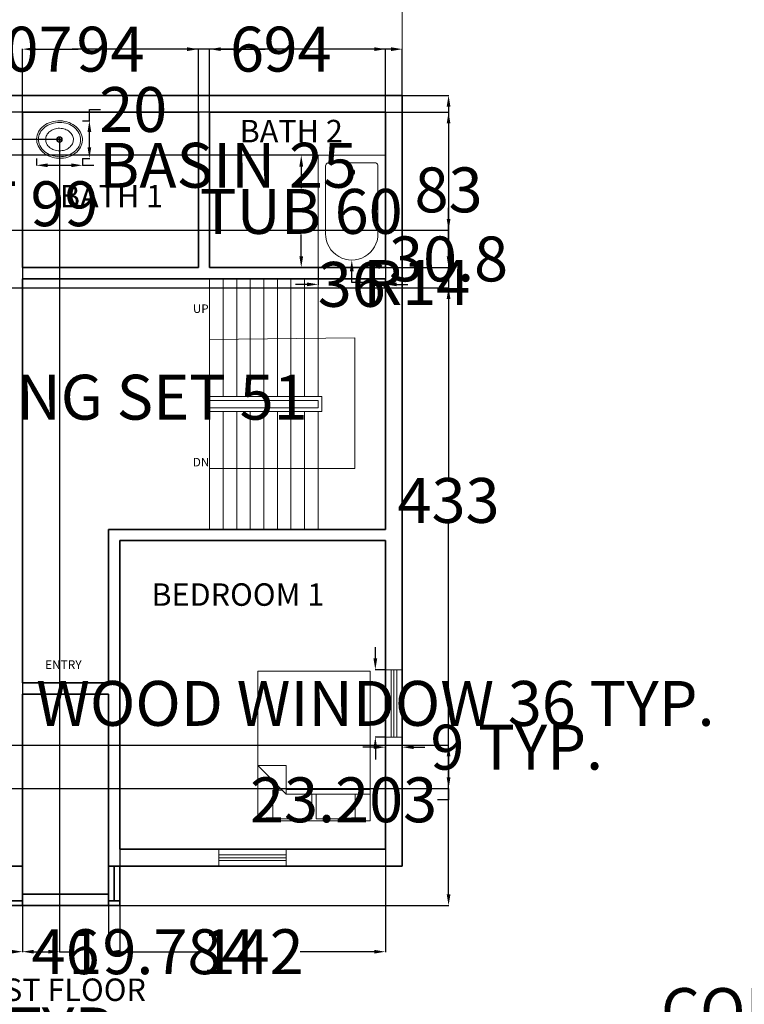
# Model space of a CAD drawing. Units: inches. Extents: x -15 to 1815, y 1023 to 2303.
# Tile 4 of 8: x 522 to 910, y 1772 to 2299. Entities that reach past the tile are written whole.
import ezdxf

# ---------------------------------------------------------------- set-up
doc = ezdxf.new("R2010")
doc.units = ezdxf.units.IN
doc.header["$MEASUREMENT"] = 0
for name, color, linetype, lineweight in [('A-ANNO-DIMS', 2, 'Continuous', 18), ('A-ANNO-TEXT', 7, 'Continuous', 25), ('A-AREA-IDEN', 7, 'Continuous', 18), ('A-FLOR-FIXT', 9, 'Continuous', 18), ('A-FLOR-STRS', 3, 'Continuous', 18), ('A-FURN', 8, 'Continuous', 18), ('A-GLAZ', 4, 'Continuous', 18), ('A-REFR', 8, 'Continuous', 13), ('A-WALL', 7, 'Continuous', 35)]:
    doc.layers.add(name, color=color, linetype=linetype, lineweight=lineweight)
doc.styles.get("Standard").update_dxf_attribs({"font": 'arial.ttf'})
doc.dimstyles.get("Standard").update_dxf_attribs({"dimtxt": 24, "dimasz": 6, "dimexe": 0.18, "dimexo": 0.0625, "dimgap": 0.09, "dimtad": 0, "dimtih": 1, "dimtoh": 1, "dimdec": 0, "dimzin": 0, "dimdsep": 46, "dimlunit": 3, "dimtxsty": 'Standard', "dimcen": 0.09, "dimadec": 0, "dimazin": 0, "dimtfac": 1, "dimtdec": 0, "dimtofl": 0, "dimtmove": 0, "dimatfit": 3, "dimfxl": 1, "dimtolj": 1, "dimtzin": 0, "dimarcsym": 0})

# ---------------------------------------------------------------- blocks, each defined once
blk = doc.blocks.new('Bed - Queen')
for p, q in [((0, -80.00003), (0, 0)), ((0, 0), (59.99999, 0)), ((59.99999, 0), (59.99999, -80.00003)), ((7.99999, -1.2), (28.79998, -1.2)), ((7.99999, -14.4), (7.99999, -1.2)), ((28.79998, -1.2), (28.79998, -14.4)), ((31.19999, -1.2), (51.99999, -1.2)), ((31.19999, -14.4), (31.19999, -1.2)), ((51.99999, -1.2), (51.99999, -16.4)), ((0, -14.4), (44.8, -14.4)), ((59.99999, -29.6), (44.8, -14.4)), ((44.8, -14.4), (44.8, -29.6)), ((44.8, -16.8), (0, -16.8)), ((51.99999, -16.4), (46.79936, -16.4)), ((44.8, -29.6), (59.99999, -29.6)), ((59.99999, -80.00003), (0, -80.00003))]:
    blk.add_line(p, q)
blk = doc.blocks.new('Bath Tub - 26 x 60 in.')
for p, q in [((8, -18), (10, -18)), ((9, -17), (9, -19))]:
    blk.add_line(p, q)
blk.add_lwpolyline([(0, -36), (0, 0), (60, 0), (60, -36)], close=True)
for points in [[(6, -4), (42, -4)], [(4, -30), (4, -6)], [(42, -32), (6, -32)]]:
    blk.add_lwpolyline(points)
for radius in [1.5, 1]:
    blk.add_circle((9, -18), radius)
for centre, radius, start, end in [((5.75, -5.75), 1.77, 81.8699, 188.1301), ((42, -18), 14, 270, 90), ((5.75, -30.25), 1.77, 171.8699, 278.1301)]:
    blk.add_arc(centre, radius, start, end)
blk = doc.blocks.new('Sink - Oval top')
for p, q in [((-1, 0), (1, 0)), ((0, 1), (0, -1))]:
    blk.add_line(p, q)
for points in [[(-12.23, 0.39, 0.117634), (-11.46, -3.36, 0.104469), (-8.88, -6.8, 0.090016), (-5.08, -9.07, 0.08192), (-0.32, -10.02, 0.08192), (4.49, -9.38, 0.090016), (8.42, -7.36, 0.104469), (11.22, -4.09, 0.117634), (12.23, -0.39, 0.117634), (11.46, 3.36, 0.104469), (8.88, 6.8, 0.090016), (5.08, 9.07, 0.08192), (0.32, 10.02, 0.08192), (-4.49, 9.38, 0.090016), (-8.42, 7.36, 0.104469), (-11.22, 4.09, 0.117634)], [(-11.29, 0.16, 0.118622), (-10.52, -3.25, 0.104678), (-8.07, -6.36, 0.089562), (-4.54, -8.37, 0.081185), (-0.13, -9.15, 0.081185), (4.3, -8.49, 0.089562), (7.89, -6.58, 0.104678), (10.42, -3.55, 0.118622), (11.29, -0.16, 0.118622), (10.52, 3.25, 0.104678), (8.07, 6.36, 0.089562), (4.54, 8.37, 0.081185), (0.13, 9.15, 0.081185), (-4.3, 8.49, 0.089562), (-7.89, 6.58, 0.104678), (-10.42, 3.55, 0.118622)], [(-7.42, 0.08, 0.118283), (-6.91, -2.17, 0.104607), (-5.29, -4.21, 0.089718), (-2.97, -5.53, 0.081436), (-0.07, -6.04, 0.081436), (2.84, -5.59, 0.089718), (5.2, -4.33, 0.104607), (6.86, -2.32, 0.118283), (7.42, -0.08, 0.118283), (6.91, 2.17, 0.104607), (5.29, 4.21, 0.089718), (2.97, 5.53, 0.081436), (0.07, 6.04, 0.081436), (-2.84, 5.59, 0.089718), (-5.2, 4.33, 0.104607), (-6.86, 2.32, 0.118283)]]:
    blk.add_lwpolyline(points, format="xyb", close=True)
for radius in [1.5, 1]:
    blk.add_circle((0, 0), radius)
blk = doc.blocks.new('Window - Wood Frame 36 in. Wide plan')
for p, q in [((0, 7.5), (0, -1.5)), ((36, 7.5), (36, -1.5)), ((0, 4.5), (36, 4.5)), ((0, 3), (36, 3)), ((0, 1.5), (36, 1.5))]:
    blk.add_line(p, q)
blk = doc.blocks.new('STAIR-RETURN-PLAN')
for p, q in [((0, 69), (0, 134)), ((7.25, 71), (7.25, 134)), ((14.5, 71), (14.5, 134)), ((21.75, 71), (21.75, 134)), ((29, 71), (29, 134)), ((36.25, 71), (36.25, 134)), ((43.5, 71), (43.5, 134)), ((50.75, 71), (50.75, 134)), ((58, 71), (58, 134)), ((58, 71), (58, 134)), ((0, 101.5), (77.56, 102.5)), ((77.56, 102.5), (77.56, 32.54)), ((60, 71), (0, 71)), ((58, 69), (0, 69)), ((58, 65), (58, 69)), ((60, 65), (60, 71)), ((58, 65), (0, 65)), ((0, 0), (0, 65)), ((60, 63), (60, 65)), ((60, 63), (0, 63)), ((7.25, 0), (7.25, 63)), ((14.5, 0), (14.5, 63)), ((21.75, 0), (21.75, 63)), ((29, 0), (29, 63)), ((36.25, 0), (36.25, 63)), ((43.5, 0), (43.5, 63)), ((50.75, 0), (50.75, 63)), ((58, 0), (58, 63)), ((58, 0), (58, 63)), ((77.56, 32.54), (0, 32.5))]:
    blk.add_line(p, q)
blk = doc.blocks.new('*D21')
at = {"layer": 'A-ANNO-DIMS', "color": 0, "lineweight": -2, "transparency": 16777216}
for p, q in [((712.43, 1957.33), (712.43, 1963.33)), ((717.77, 1951.33), (712.25, 1951.33)), ((717.77, 1915.33), (712.25, 1915.33)), ((712.43, 1909.33), (712.43, 1903.33))]:
    blk.add_line(p, q, dxfattribs=at)
at = {"layer": 'A-ANNO-DIMS', "color": 0, "transparency": 16777216}
for points in [[(711.43, 1957.33), (713.43, 1957.33), (712.43, 1951.33)], [(711.43, 1909.33), (713.43, 1909.33), (712.43, 1915.33)]]:
    blk.add_solid(points, dxfattribs=at)
at = {"layer": 'Defpoints', "color": 0, "transparency": 16777216}
for p in [(717.83, 1951.33), (712.43, 1915.33), (717.83, 1915.33)]:
    blk.add_point(p, dxfattribs=at)
at = {"layer": 'A-ANNO-DIMS', "color": 0, "transparency": 16777216, "insert": (712.43, 1933.33), "char_height": 24, "attachment_point": 5}
blk.add_mtext('\\A1;WOOD WINDOW 36 TYP.', dxfattribs=at)
blk = doc.blocks.new('*D22')
at = {"layer": 'A-ANNO-DIMS', "color": 0, "lineweight": -2, "transparency": 16777216}
for p, q in [((717.83, 1915.26), (717.83, 1909.75)), ((726.83, 1915.26), (726.83, 1909.75)), ((711.83, 1909.93), (705.83, 1909.93)), ((732.83, 1909.93), (738.83, 1909.93))]:
    blk.add_line(p, q, dxfattribs=at)
at = {"layer": 'A-ANNO-DIMS', "color": 0, "transparency": 16777216}
for points in [[(711.83, 1910.93), (711.83, 1908.93), (717.83, 1909.93)], [(732.83, 1910.93), (732.83, 1908.93), (726.83, 1909.93)]]:
    blk.add_solid(points, dxfattribs=at)
at = {"layer": 'Defpoints', "color": 0, "transparency": 16777216}
for p in [(717.83, 1915.33), (726.83, 1915.33), (726.83, 1909.93)]:
    blk.add_point(p, dxfattribs=at)
at = {"layer": 'A-ANNO-DIMS', "color": 0, "transparency": 16777216, "insert": (788.01, 1909.93), "char_height": 24, "attachment_point": 5}
blk.add_mtext('\\A1;9 TYP.', dxfattribs=at)
blk = doc.blocks.new('*D33')
at = {"layer": 'A-ANNO-DIMS', "color": 0, "lineweight": -2, "transparency": 16777216}
for p, q in [((393.59, 2104.63), (393.59, 2096.83)), ((444.77, 2104.63), (444.77, 2096.83)), ((399.59, 2097.01), (438.77, 2097.01)), ((444.77, 2097.01), (450.77, 2097.01))]:
    blk.add_line(p, q, dxfattribs=at)
at = {"layer": 'A-ANNO-DIMS', "color": 0, "transparency": 16777216}
for points in [[(399.59, 2098.01), (399.59, 2096.01), (393.59, 2097.01)], [(438.77, 2098.01), (438.77, 2096.01), (444.77, 2097.01)]]:
    blk.add_solid(points, dxfattribs=at)
at = {"layer": 'Defpoints', "color": 0, "transparency": 16777216}
for p in [(393.59, 2104.69), (444.77, 2104.69), (444.77, 2097.01)]:
    blk.add_point(p, dxfattribs=at)
at = {"layer": 'A-ANNO-DIMS', "color": 0, "transparency": 16777216, "insert": (565.73, 2097.01), "char_height": 24, "attachment_point": 5}
blk.add_mtext('\\A1;DINING SET 51', dxfattribs=at)
blk = doc.blocks.new('*D35')
at = {"layer": 'A-ANNO-DIMS', "color": 0, "lineweight": -2, "transparency": 16777216}
for p, q in [((681.77, 2226.33), (672.65, 2226.33)), ((672.83, 2220.33), (672.83, 2208.67)), ((672.83, 2172.33), (672.83, 2183.98)), ((681.77, 2166.33), (672.65, 2166.33))]:
    blk.add_line(p, q, dxfattribs=at)
at = {"layer": 'A-ANNO-DIMS', "color": 0, "transparency": 16777216}
for points in [[(671.83, 2220.33), (673.83, 2220.33), (672.83, 2226.33)], [(671.83, 2172.33), (673.83, 2172.33), (672.83, 2166.33)]]:
    blk.add_solid(points, dxfattribs=at)
at = {"layer": 'Defpoints', "color": 0, "transparency": 16777216}
for p in [(681.83, 2226.33), (672.83, 2166.33), (681.83, 2166.33)]:
    blk.add_point(p, dxfattribs=at)
at = {"layer": 'A-ANNO-DIMS', "color": 0, "transparency": 16777216, "insert": (672.83, 2196.33), "char_height": 24, "attachment_point": 5}
blk.add_mtext('\\A1;TUB 60', dxfattribs=at)
blk = doc.blocks.new('*D36')
at = {"layer": 'A-ANNO-DIMS', "color": 0, "lineweight": -2, "transparency": 16777216}
for p, q in [((681.83, 2166.26), (681.83, 2157.15)), ((717.83, 2166.26), (717.83, 2157.15)), ((675.83, 2157.33), (669.83, 2157.33)), ((723.83, 2157.33), (729.83, 2157.33))]:
    blk.add_line(p, q, dxfattribs=at)
at = {"layer": 'A-ANNO-DIMS', "color": 0, "transparency": 16777216}
for points in [[(675.83, 2158.33), (675.83, 2156.33), (681.83, 2157.33)], [(723.83, 2158.33), (723.83, 2156.33), (717.83, 2157.33)]]:
    blk.add_solid(points, dxfattribs=at)
at = {"layer": 'Defpoints', "color": 0, "transparency": 16777216}
for p in [(681.83, 2166.33), (717.83, 2166.33), (717.83, 2157.33)]:
    blk.add_point(p, dxfattribs=at)
at = {"layer": 'A-ANNO-DIMS', "color": 0, "transparency": 16777216, "insert": (699.83, 2157.33), "char_height": 24, "attachment_point": 5}
blk.add_mtext('\\A1;36', dxfattribs=at)
blk = doc.blocks.new('*D37')
at = {"layer": 'A-ANNO-DIMS', "color": 0, "lineweight": -2, "transparency": 16777216}
for p, q in [((531.34, 2224.6), (531.34, 2220.8)), ((555.89, 2224.6), (555.89, 2220.8)), ((537.34, 2220.98), (549.89, 2220.98)), ((555.89, 2220.98), (561.89, 2220.98))]:
    blk.add_line(p, q, dxfattribs=at)
at = {"layer": 'A-ANNO-DIMS', "color": 0, "transparency": 16777216}
for points in [[(537.34, 2221.98), (537.34, 2219.98), (531.34, 2220.98)], [(549.89, 2221.98), (549.89, 2219.98), (555.89, 2220.98)]]:
    blk.add_solid(points, dxfattribs=at)
at = {"layer": 'Defpoints', "color": 0, "transparency": 16777216}
for p in [(531.34, 2224.66), (555.89, 2224.66), (555.89, 2220.98)]:
    blk.add_point(p, dxfattribs=at)
at = {"layer": 'A-ANNO-DIMS', "color": 0, "transparency": 16777216, "insert": (633.7, 2220.98), "char_height": 24, "attachment_point": 5}
blk.add_mtext('\\A1;BASIN 25', dxfattribs=at)
blk = doc.blocks.new('*D38')
at = {"layer": 'A-ANNO-DIMS', "color": 0, "lineweight": -2, "transparency": 16777216}
for p, q in [((559.58, 2244.8), (559.58, 2250.8)), ((559.58, 2250.8), (565.58, 2250.8)), ((555.96, 2244.8), (559.76, 2244.8)), ((559.58, 2230.66), (559.58, 2238.8)), ((555.96, 2224.66), (559.76, 2224.66))]:
    blk.add_line(p, q, dxfattribs=at)
at = {"layer": 'A-ANNO-DIMS', "color": 0, "transparency": 16777216}
for points in [[(558.58, 2238.8), (560.58, 2238.8), (559.58, 2244.8)], [(558.58, 2230.66), (560.58, 2230.66), (559.58, 2224.66)]]:
    blk.add_solid(points, dxfattribs=at)
at = {"layer": 'Defpoints', "color": 0, "transparency": 16777216}
for p in [(555.89, 2244.8), (559.58, 2244.8), (555.89, 2224.66)]:
    blk.add_point(p, dxfattribs=at)
at = {"layer": 'A-ANNO-DIMS', "color": 0, "transparency": 16777216, "insert": (583.02, 2250.8), "char_height": 24, "attachment_point": 5}
blk.add_mtext('\\A1;20', dxfattribs=at)
blk = doc.blocks.new('*D39')
at = {"layer": 'A-ANNO-DIMS', "color": 0, "lineweight": -2, "transparency": 16777216}
for p, q in [((416.85, 2250.01), (431.85, 2250.01)), ((431.67, 2244.01), (431.67, 2212.92)), ((431.67, 2156.83), (431.67, 2187.92)), ((416.85, 2150.83), (431.85, 2150.83))]:
    blk.add_line(p, q, dxfattribs=at)
at = {"layer": 'A-ANNO-DIMS', "color": 0, "transparency": 16777216}
for points in [[(430.67, 2244.01), (432.67, 2244.01), (431.67, 2250.01)], [(430.67, 2156.83), (432.67, 2156.83), (431.67, 2150.83)]]:
    blk.add_solid(points, dxfattribs=at)
at = {"layer": 'Defpoints', "color": 0, "transparency": 16777216}
for p in [(416.79, 2250.01), (431.67, 2250.01), (416.79, 2150.83)]:
    blk.add_point(p, dxfattribs=at)
at = {"layer": 'A-ANNO-DIMS', "color": 0, "transparency": 16777216, "insert": (431.67, 2200.42), "char_height": 24, "attachment_point": 5}
blk.add_mtext('\\A1;KITCHEN UNIT 99', dxfattribs=at)
blk = doc.blocks.new('*D45')
at = {"layer": 'A-ANNO-DIMS', "color": 0, "lineweight": -2, "transparency": 16777216}
for p, q in [((1138.43, 1769.16), (1132.43, 1769.16)), ((1138.43, 1750.02), (1138.43, 1769.34)), ((1260.44, 1769.16), (1144.43, 1769.16)), ((1266.44, 1750.02), (1266.44, 1769.34))]:
    blk.add_line(p, q, dxfattribs=at)
at = {"layer": 'A-ANNO-DIMS', "color": 0, "transparency": 16777216}
for points in [[(1144.43, 1770.16), (1144.43, 1768.16), (1138.43, 1769.16)], [(1260.44, 1770.16), (1260.44, 1768.16), (1266.44, 1769.16)]]:
    blk.add_solid(points, dxfattribs=at)
at = {"layer": 'Defpoints', "color": 0, "transparency": 16777216}
for p in [(1138.43, 1769.16), (1138.43, 1749.96), (1266.44, 1749.96)]:
    blk.add_point(p, dxfattribs=at)
at = {"layer": 'A-ANNO-DIMS', "color": 0, "transparency": 16777216, "insert": (993.96, 1769.16), "char_height": 24, "attachment_point": 5}
blk.add_mtext('\\A1;COPING 128 TYP.', dxfattribs=at)
blk = doc.blocks.new('*D57')
at = {"layer": 'A-ANNO-DIMS', "color": 0, "lineweight": -2, "transparency": 16777216}
for p, q in [((317.89, 1716.39), (317.89, 1758.98)), ((323.89, 1758.8), (327.1, 1758.8)), ((595.01, 1758.8), (591.8, 1758.8)), ((601.01, 1716.39), (601.01, 1758.98))]:
    blk.add_line(p, q, dxfattribs=at)
at = {"layer": 'A-ANNO-DIMS', "color": 0, "transparency": 16777216}
for points in [[(323.89, 1759.8), (323.89, 1757.8), (317.89, 1758.8)], [(595.01, 1759.8), (595.01, 1757.8), (601.01, 1758.8)]]:
    blk.add_solid(points, dxfattribs=at)
at = {"layer": 'Defpoints', "color": 0, "transparency": 16777216}
for p in [(601.01, 1758.8), (317.89, 1716.33), (601.01, 1716.33)]:
    blk.add_point(p, dxfattribs=at)
at = {"layer": 'A-ANNO-DIMS', "color": 0, "transparency": 16777216, "insert": (459.45, 1758.8), "char_height": 24, "attachment_point": 5}
blk.add_mtext('\\A1;FASCIA 283 TYP.', dxfattribs=at)
blk = doc.blocks.new('*D59')
at = {"layer": 'A-ANNO-DIMS', "color": 0, "lineweight": -2, "transparency": 16777216}
for p, q in [((319.83, 2258.39), (319.83, 2283.24)), ((325.83, 2283.06), (496.25, 2283.06)), ((720.83, 2283.06), (550.42, 2283.06)), ((726.83, 2258.39), (726.83, 2283.24))]:
    blk.add_line(p, q, dxfattribs=at)
at = {"layer": 'A-ANNO-DIMS', "color": 0, "transparency": 16777216}
for points in [[(325.83, 2284.06), (325.83, 2282.06), (319.83, 2283.06)], [(720.83, 2284.06), (720.83, 2282.06), (726.83, 2283.06)]]:
    blk.add_solid(points, dxfattribs=at)
at = {"layer": 'Defpoints', "color": 0, "transparency": 16777216}
for p in [(726.83, 2283.06), (319.83, 2258.33), (726.83, 2258.33)]:
    blk.add_point(p, dxfattribs=at)
at = {"layer": 'A-ANNO-DIMS', "color": 0, "transparency": 16777216, "insert": (523.33, 2283.06), "char_height": 24, "attachment_point": 5}
blk.add_mtext('\\A1;407', dxfattribs=at)
blk = doc.blocks.new('*D60')
at = {"layer": 'A-ANNO-DIMS', "color": 0, "lineweight": -2, "transparency": 16777216}
for p, q in [((726.9, 2258.33), (751.75, 2258.33)), ((751.57, 2252.33), (751.57, 2054.18)), ((751.57, 1831.33), (751.57, 2029.48)), ((575.9, 1825.33), (751.75, 1825.33))]:
    blk.add_line(p, q, dxfattribs=at)
at = {"layer": 'A-ANNO-DIMS', "color": 0, "transparency": 16777216}
for points in [[(750.57, 2252.33), (752.57, 2252.33), (751.57, 2258.33)], [(750.57, 1831.33), (752.57, 1831.33), (751.57, 1825.33)]]:
    blk.add_solid(points, dxfattribs=at)
at = {"layer": 'Defpoints', "color": 0, "transparency": 16777216}
for p in [(726.83, 2258.33), (575.83, 1825.33), (751.57, 1825.33)]:
    blk.add_point(p, dxfattribs=at)
at = {"layer": 'A-ANNO-DIMS', "color": 0, "transparency": 16777216, "insert": (751.57, 2041.83), "char_height": 24, "attachment_point": 5}
blk.add_mtext('\\A1;433', dxfattribs=at)
blk = doc.blocks.new('*D64')
at = {"layer": 'A-ANNO-DIMS', "color": 0, "lineweight": -2, "transparency": 16777216}
for p, q in [((523.834675, 1846.264776), (523.834675, 1800.414776)), ((569.834675, 1846.264776), (569.834675, 1800.414776)), ((517.834675, 1800.594776), (511.834675, 1800.594776)), ((575.834675, 1800.594776), (581.834675, 1800.594776))]:
    blk.add_line(p, q, dxfattribs=at)
at = {"layer": 'A-ANNO-DIMS', "color": 0, "transparency": 16777216}
for points in [[(517.834675, 1801.594776), (517.834675, 1799.594776), (523.834675, 1800.594776)], [(575.834675, 1801.594776), (575.834675, 1799.594776), (569.834675, 1800.594776)]]:
    blk.add_solid(points, dxfattribs=at)
at = {"layer": 'Defpoints', "color": 0, "transparency": 16777216}
for p in [(523.834675, 1846.327276), (569.834675, 1846.327276), (569.834675, 1800.594776)]:
    blk.add_point(p, dxfattribs=at)
at = {"layer": 'A-ANNO-DIMS', "color": 0, "transparency": 16777216, "insert": (546.834675, 1800.594776), "char_height": 24, "attachment_point": 5}
blk.add_mtext('\\A1;46', dxfattribs=at)
blk = doc.blocks.new('*D65')
at = {"layer": 'A-ANNO-DIMS', "color": 0, "lineweight": -2, "transparency": 16777216}
for p, q in [((575.83, 1855.26), (575.83, 1800.41)), ((717.83, 1855.26), (717.83, 1800.41)), ((581.83, 1800.59), (621.48, 1800.59)), ((711.83, 1800.59), (672.19, 1800.59))]:
    blk.add_line(p, q, dxfattribs=at)
at = {"layer": 'A-ANNO-DIMS', "color": 0, "transparency": 16777216}
for points in [[(581.83, 1801.59), (581.83, 1799.59), (575.83, 1800.59)], [(711.83, 1801.59), (711.83, 1799.59), (717.83, 1800.59)]]:
    blk.add_solid(points, dxfattribs=at)
at = {"layer": 'Defpoints', "color": 0, "transparency": 16777216}
for p in [(575.83, 1855.33), (717.83, 1855.33), (717.83, 1800.59)]:
    blk.add_point(p, dxfattribs=at)
at = {"layer": 'A-ANNO-DIMS', "color": 0, "transparency": 16777216, "insert": (646.83, 1800.59), "char_height": 24, "attachment_point": 5}
blk.add_mtext('\\A1;142', dxfattribs=at)
blk = doc.blocks.new('*D69')
at = {"layer": 'A-ANNO-DIMS', "color": 0, "lineweight": -2, "transparency": 16777216}
for p, q in [((407.38, 1910.99), (751.75, 1910.99)), ((751.57, 1904.99), (751.57, 1893.79)), ((420.46, 1887.79), (751.75, 1887.79)), ((751.57, 1887.79), (751.57, 1881.79)), ((751.57, 1881.79), (745.57, 1881.79))]:
    blk.add_line(p, q, dxfattribs=at)
at = {"layer": 'A-ANNO-DIMS', "color": 0, "transparency": 16777216}
for points in [[(750.57, 1904.99), (752.57, 1904.99), (751.57, 1910.99)], [(750.57, 1893.79), (752.57, 1893.79), (751.57, 1887.79)]]:
    blk.add_solid(points, dxfattribs=at)
at = {"layer": 'Defpoints', "color": 0, "transparency": 16777216}
for p in [(407.31, 1910.99), (420.39, 1887.79), (751.57, 1887.79)]:
    blk.add_point(p, dxfattribs=at)
at = {"layer": 'A-ANNO-DIMS', "color": 0, "transparency": 16777216, "insert": (695.46, 1881.79), "char_height": 24, "attachment_point": 5}
blk.add_mtext('\\A1;23.203', dxfattribs=at)
blk = doc.blocks.new('*D70')
at = {"layer": 'A-ANNO-DIMS', "color": 0, "lineweight": -2, "transparency": 16777216}
for p, q in [((523.83, 2249.39), (523.83, 2283.24)), ((529.83, 2283.06), (553.6, 2283.06)), ((611.83, 2283.06), (588.07, 2283.06)), ((617.83, 2249.39), (617.83, 2283.24))]:
    blk.add_line(p, q, dxfattribs=at)
at = {"layer": 'A-ANNO-DIMS', "color": 0, "transparency": 16777216}
for points in [[(529.83, 2284.06), (529.83, 2282.06), (523.83, 2283.06)], [(611.83, 2284.06), (611.83, 2282.06), (617.83, 2283.06)]]:
    blk.add_solid(points, dxfattribs=at)
at = {"layer": 'Defpoints', "color": 0, "transparency": 16777216}
for p in [(617.83, 2283.06), (523.83, 2249.33), (617.83, 2249.33)]:
    blk.add_point(p, dxfattribs=at)
at = {"layer": 'A-ANNO-DIMS', "color": 0, "transparency": 16777216, "insert": (570.83, 2283.06), "char_height": 24, "attachment_point": 5}
blk.add_mtext('\\A1;94', dxfattribs=at)
blk = doc.blocks.new('*D71')
at = {"layer": 'A-ANNO-DIMS', "color": 0, "lineweight": -2, "transparency": 16777216}
for p, q in [((623.83, 2249.39), (623.83, 2283.24)), ((629.83, 2283.06), (653.6, 2283.06)), ((711.83, 2283.06), (688.07, 2283.06)), ((717.83, 2249.39), (717.83, 2283.24))]:
    blk.add_line(p, q, dxfattribs=at)
at = {"layer": 'A-ANNO-DIMS', "color": 0, "transparency": 16777216}
for points in [[(629.83, 2284.06), (629.83, 2282.06), (623.83, 2283.06)], [(711.83, 2284.06), (711.83, 2282.06), (717.83, 2283.06)]]:
    blk.add_solid(points, dxfattribs=at)
at = {"layer": 'Defpoints', "color": 0, "transparency": 16777216}
for p in [(717.83, 2283.06), (623.83, 2249.33), (717.83, 2249.33)]:
    blk.add_point(p, dxfattribs=at)
at = {"layer": 'A-ANNO-DIMS', "color": 0, "transparency": 16777216, "insert": (670.83, 2283.06), "char_height": 24, "attachment_point": 5}
blk.add_mtext('\\A1;94', dxfattribs=at)
blk = doc.blocks.new('*D72')
at = {"layer": 'A-ANNO-DIMS', "color": 0, "lineweight": -2, "transparency": 16777216}
for p, q in [((611.83, 2283.06), (605.83, 2283.06)), ((617.83, 2249.39), (617.83, 2283.24)), ((623.83, 2249.39), (623.83, 2283.24)), ((629.83, 2283.06), (635.83, 2283.06))]:
    blk.add_line(p, q, dxfattribs=at)
at = {"layer": 'A-ANNO-DIMS', "color": 0, "transparency": 16777216}
for points in [[(611.83, 2284.06), (611.83, 2282.06), (617.83, 2283.06)], [(629.83, 2284.06), (629.83, 2282.06), (623.83, 2283.06)]]:
    blk.add_solid(points, dxfattribs=at)
at = {"layer": 'Defpoints', "color": 0, "transparency": 16777216}
for p in [(623.83, 2283.06), (617.83, 2249.33), (623.83, 2249.33)]:
    blk.add_point(p, dxfattribs=at)
at = {"layer": 'A-ANNO-DIMS', "color": 0, "transparency": 16777216, "insert": (643.85, 2283.06), "char_height": 24, "attachment_point": 5}
blk.add_mtext('\\A1;6', dxfattribs=at)
blk = doc.blocks.new('*D73')
at = {"layer": 'A-ANNO-DIMS', "color": 0, "lineweight": -2, "transparency": 16777216}
for p, q in [((717.9, 2249.33), (751.75, 2249.33)), ((751.57, 2243.33), (751.57, 2220.18)), ((751.57, 2172.33), (751.57, 2195.48)), ((717.9, 2166.33), (751.75, 2166.33))]:
    blk.add_line(p, q, dxfattribs=at)
at = {"layer": 'A-ANNO-DIMS', "color": 0, "transparency": 16777216}
for points in [[(750.57, 2243.33), (752.57, 2243.33), (751.57, 2249.33)], [(750.57, 2172.33), (752.57, 2172.33), (751.57, 2166.33)]]:
    blk.add_solid(points, dxfattribs=at)
at = {"layer": 'Defpoints', "color": 0, "transparency": 16777216}
for p in [(717.83, 2249.33), (751.57, 2249.33), (717.83, 2166.33)]:
    blk.add_point(p, dxfattribs=at)
at = {"layer": 'A-ANNO-DIMS', "color": 0, "transparency": 16777216, "insert": (751.57, 2207.83), "char_height": 24, "attachment_point": 5}
blk.add_mtext('\\A1;83', dxfattribs=at)
blk = doc.blocks.new('*D74')
at = {"layer": 'A-ANNO-DIMS', "color": 0, "lineweight": -2, "transparency": 16777216}
for p, q in [((295.1, 2249.33), (295.1, 2255.33)), ((295.1, 2255.33), (301.1, 2255.33)), ((623.77, 2249.33), (294.92, 2249.33)), ((295.1, 2232.33), (295.1, 2243.33)), ((681.77, 2226.33), (294.92, 2226.33))]:
    blk.add_line(p, q, dxfattribs=at)
at = {"layer": 'A-ANNO-DIMS', "color": 0, "transparency": 16777216}
for points in [[(294.1, 2243.33), (296.1, 2243.33), (295.1, 2249.33)], [(294.1, 2232.33), (296.1, 2232.33), (295.1, 2226.33)]]:
    blk.add_solid(points, dxfattribs=at)
at = {"layer": 'Defpoints', "color": 0, "transparency": 16777216}
for p in [(295.1, 2249.33), (623.83, 2249.33), (681.83, 2226.33)]:
    blk.add_point(p, dxfattribs=at)
at = {"layer": 'A-ANNO-DIMS', "color": 0, "transparency": 16777216, "insert": (318.59, 2255.33), "char_height": 24, "attachment_point": 5}
blk.add_mtext('\\A1;23', dxfattribs=at)
blk = doc.blocks.new('*D75')
at = {"layer": 'A-ANNO-DIMS', "color": 0, "lineweight": -2, "transparency": 16777216}
for p, q in [((523.83, 2249.26), (523.83, 1800.41)), ((543.62, 2234.67), (543.62, 1800.41)), ((529.83, 1800.59), (537.62, 1800.59)), ((543.62, 1800.59), (549.62, 1800.59))]:
    blk.add_line(p, q, dxfattribs=at)
at = {"layer": 'A-ANNO-DIMS', "color": 0, "transparency": 16777216}
for points in [[(529.83, 1801.59), (529.83, 1799.59), (523.83, 1800.59)], [(537.62, 1801.59), (537.62, 1799.59), (543.62, 1800.59)]]:
    blk.add_solid(points, dxfattribs=at)
at = {"layer": 'Defpoints', "color": 0, "transparency": 16777216}
for p in [(523.83, 2249.33), (543.62, 2234.73), (543.62, 1800.59)]:
    blk.add_point(p, dxfattribs=at)
at = {"layer": 'A-ANNO-DIMS', "color": 0, "transparency": 16777216, "insert": (598.35, 1800.59), "char_height": 24, "attachment_point": 5}
blk.add_mtext('\\A1;19.784', dxfattribs=at)
blk = doc.blocks.new('*D76')
at = {"layer": 'A-ANNO-DIMS', "color": 0, "lineweight": -2, "transparency": 16777216}
for p, q in [((523.77, 2249.33), (294.92, 2249.33)), ((295.1, 2243.33), (295.1, 2240.73)), ((543.56, 2234.73), (294.92, 2234.73)), ((295.1, 2234.73), (295.1, 2228.73)), ((295.1, 2228.73), (289.1, 2228.73))]:
    blk.add_line(p, q, dxfattribs=at)
at = {"layer": 'A-ANNO-DIMS', "color": 0, "transparency": 16777216}
for points in [[(294.1, 2243.33), (296.1, 2243.33), (295.1, 2249.33)], [(294.1, 2240.73), (296.1, 2240.73), (295.1, 2234.73)]]:
    blk.add_solid(points, dxfattribs=at)
at = {"layer": 'Defpoints', "color": 0, "transparency": 16777216}
for p in [(523.83, 2249.33), (295.1, 2234.73), (543.62, 2234.73)]:
    blk.add_point(p, dxfattribs=at)
at = {"layer": 'A-ANNO-DIMS', "color": 0, "transparency": 16777216, "insert": (240.33, 2228.73), "char_height": 24, "attachment_point": 5}
blk.add_mtext('\\A1;14.596', dxfattribs=at)
blk = doc.blocks.new('*D79')
at = {"layer": 'A-ANNO-DIMS', "color": 0, "lineweight": -2, "transparency": 16777216}
for p, q in [((751.57, 2192.31), (751.57, 2198.31)), ((392.63, 2186.31), (751.75, 2186.31)), ((412.17, 2155.51), (751.75, 2155.51)), ((751.57, 2149.51), (751.57, 2143.51))]:
    blk.add_line(p, q, dxfattribs=at)
at = {"layer": 'A-ANNO-DIMS', "color": 0, "transparency": 16777216}
for points in [[(750.57, 2192.31), (752.57, 2192.31), (751.57, 2186.31)], [(750.57, 2149.51), (752.57, 2149.51), (751.57, 2155.51)]]:
    blk.add_solid(points, dxfattribs=at)
at = {"layer": 'Defpoints', "color": 0, "transparency": 16777216}
for p in [(392.57, 2186.31), (412.11, 2155.51), (751.57, 2155.51)]:
    blk.add_point(p, dxfattribs=at)
at = {"layer": 'A-ANNO-DIMS', "color": 0, "transparency": 16777216, "insert": (751.57, 2170.91), "char_height": 24, "attachment_point": 5}
blk.add_mtext('\\A1;30.8', dxfattribs=at)
blk = doc.blocks.new('*D128')
at = {"layer": 'A-ANNO-DIMS', "color": 0, "lineweight": -2, "transparency": 16777216}
for p, q in [((699.74, 2184.33), (699.92, 2184.33)), ((699.83, 2184.24), (699.83, 2184.42)), ((699.84, 2158.33), (699.84, 2164.33)), ((705.84, 2158.33), (699.84, 2158.33))]:
    blk.add_line(p, q, dxfattribs=at)
at = {"layer": 'A-ANNO-DIMS', "color": 0, "transparency": 16777216}
blk.add_solid([(700.84, 2164.33), (698.84, 2164.33), (699.84, 2170.33)], dxfattribs=at)
at = {"layer": 'Defpoints', "color": 0, "transparency": 16777216}
for p in [(699.83, 2184.33), (699.84, 2170.33)]:
    blk.add_point(p, dxfattribs=at)
at = {"layer": 'A-ANNO-DIMS', "color": 0, "transparency": 16777216, "insert": (734.55, 2158.33), "char_height": 24, "attachment_point": 5}
blk.add_mtext('\\A1;R14', dxfattribs=at)

msp = doc.modelspace()

# ---------------------------------------------------------------- linework, layer by layer
at = {"layer": 'A-REFR'}
msp.add_ray((726.8347, 1846.3273), (0, 1), dxfattribs=at)
at = {"layer": 'A-WALL'}
for p, q in [((726.8347, 2258.3273), (319.8347, 2258.3273)), ((523.8347, 2258.3273), (617.8347, 2258.3273)), ((726.8347, 1846.3273), (726.8347, 2258.3273)), ((523.8347, 2249.3273), (617.8347, 2249.3273)), ((523.8347, 2166.3273), (523.8347, 2249.3273)), ((617.8347, 2249.3273), (617.8347, 2166.3273)), ((623.8347, 2249.3273), (717.8347, 2249.3273)), ((623.8347, 2166.3273), (623.8347, 2249.3273)), ((717.8347, 2249.3273), (717.8347, 2166.3273)), ((617.8347, 2166.3273), (523.8347, 2166.3273)), ((717.8347, 2166.3273), (623.8347, 2166.3273)), ((523.8347, 2160.3273), (523.8347, 1944.3273)), ((717.8347, 2160.3273), (523.8347, 2160.3273)), ((523.8347, 2160.3273), (617.8347, 2160.3273)), ((717.8347, 2026.3273), (717.8347, 2160.3273)), ((726.8347, 2160.3273), (726.8347, 1846.3273)), ((569.8347, 2026.3273), (717.8347, 2026.3273)), ((569.8347, 2026.3273), (569.8347, 1944.3273)), ((575.8347, 2020.3273), (575.8347, 1855.3273)), ((717.8347, 2020.3273), (575.8347, 2020.3273)), ((623.8347, 2020.3273), (623.8347, 2020.3273)), ((717.8347, 1855.3273), (717.8347, 2020.3273)), ((726.8347, 1846.3273), (726.8347, 2020.3273)), ((523.8347, 1944.3273), (569.8347, 1944.3273)), ((523.8347, 1938.3273), (569.8347, 1938.3273)), ((523.8347, 1938.3273), (523.8347, 1825.3273)), ((569.8347, 1938.3273), (569.8347, 1846.3273)), ((569.8347, 1831.3273), (569.8347, 1938.3273)), ((575.8347, 1855.3273), (717.8347, 1855.3273)), ((326.8347, 1846.3273), (523.8347, 1846.3273)), ((523.8347, 1825.3273), (523.8347, 1846.3273)), ((569.8347, 1846.3273), (726.8347, 1846.3273)), ((572.8347, 1846.3273), (572.8347, 1827.7829)), ((575.8347, 1825.3273), (575.8347, 1846.3273)), ((523.8347, 1827.7829), (517.8347, 1827.7829)), ((569.8347, 1831.3273), (523.8347, 1831.3273)), ((569.8347, 1831.3273), (569.8347, 1825.3273)), ((575.8347, 1827.7829), (569.8347, 1827.7829)), ((575.8347, 1825.3273), (517.8347, 1825.3273))]:
    msp.add_line(p, q, dxfattribs=at)

# ---------------------------------------------------------------- block references
at = {"layer": 'A-FLOR-FIXT'}
msp.add_blockref('Sink - Oval top', (543.6189, 2234.7313), dxfattribs=at)
at = {"layer": 'A-FLOR-FIXT', "rotation": 270}
msp.add_blockref('Bath Tub - 26 x 60 in.', (717.8347, 2226.3273), dxfattribs=at)
at = {"layer": 'A-FLOR-STRS'}
msp.add_blockref('STAIR-RETURN-PLAN', (623.8347, 2026.3273), dxfattribs=at)
at = {"layer": 'A-FURN', "rotation": 180}
msp.add_blockref('Bed - Queen', (709.6368, 1870.4858), dxfattribs=at)
at = {"layer": 'A-GLAZ'}
for p, rotation in [((719.3347, 1951.3273), 270.0000000000001), ((664.8347, 1853.8273), 180)]:
    msp.add_blockref('Window - Wood Frame 36 in. Wide plan', p, dxfattribs=dict(at, rotation=rotation))

# ---------------------------------------------------------------- texts
at = {"layer": 'A-ANNO-TEXT'}
for s, height, p in [('UP', 4.53138, (614.9315, 2142.0504)), ('DN', 4.53138, (614.9315, 2060.0199)), ('FLOOR PLAN - FIRST FLOOR', 12, (379.3855, 1774.2654))]:
    msp.add_text(s, height=height, dxfattribs=at).set_placement(p)
at = {"layer": 'A-AREA-IDEN'}
for s, height, p in [('BATH 2 ', 12, (639.8805, 2233.2558)), ('BATH 1', 12, (543.8163, 2198.4717)), ('BEDROOM 1', 12, (592.747, 1985.4981)), ('ENTRY   ', 4.65296, (535.8983, 1951.7169))]:
    msp.add_text(s, height=height, dxfattribs=at).set_placement(p)

# ---------------------------------------------------------------- dimensions: what is measured, and where the dimension line sits
at = {"layer": 'A-ANNO-DIMS'}
for base, p1, p2, override, picture, middle in [((726.8347, 2283.0598), (319.8347, 2258.3273), (726.8347, 2258.3273), {"dimdec": 0, "dimlfac": 1, "dimrnd": 0, "dimzin": 0, "dimdsep": 46, "dimlunit": 2}, '*D59', (523.3347, 2283.0598)), ((617.8347, 2283.0598), (523.8347, 2249.3273), (617.8347, 2249.3273), {"dimdec": 0, "dimlfac": 1, "dimrnd": 0, "dimzin": 0, "dimdsep": 46, "dimlunit": 2}, '*D70', (570.8347, 2283.0598)), ((623.8347, 2283.0598), (617.8347, 2249.3273), (623.8347, 2249.3273), {"dimdec": 0, "dimlfac": 1, "dimrnd": 0, "dimzin": 0, "dimdsep": 46, "dimlunit": 2}, '*D72', (643.8483, 2283.0598)), ((717.8347, 2283.0598), (623.8347, 2249.3273), (717.8347, 2249.3273), {"dimdec": 0, "dimlfac": 1, "dimrnd": 0, "dimzin": 0, "dimdsep": 46, "dimlunit": 2}, '*D71', (670.8347, 2283.0598)), ((543.6189, 1800.5948), (523.8347, 2249.3273), (543.6189, 2234.7313), {"dimdec": 3, "dimlfac": 1, "dimrnd": 0, "dimzin": 0, "dimdsep": 46, "dimlunit": 2}, '*D75', (598.3474, 1800.5948)), ((717.8347, 2157.3273), (681.8347, 2166.3273), (717.8347, 2166.3273), {"dimdec": 0, "dimlfac": 1, "dimrnd": 0, "dimzin": 0, "dimdsep": 46, "dimlunit": 2}, '*D36', (699.8347, 2157.3273)), ((717.8347, 1800.5948), (575.8347, 1855.3273), (717.8347, 1855.3273), {"dimdec": 0, "dimlfac": 1, "dimrnd": 0, "dimzin": 0, "dimdsep": 46, "dimlunit": 2}, '*D65', (646.8347, 1800.5948)), ((569.8347, 1800.5948), (523.8347, 1846.3273), (569.8347, 1846.3273), {"dimdec": 0, "dimlfac": 1, "dimrnd": 0, "dimzin": 0, "dimdsep": 46, "dimlunit": 2}, '*D64', (546.8347, 1800.5948))]:
    dim = msp.add_linear_dim(base=base, p1=p1, p2=p2, dimstyle='Standard', override=override, dxfattribs=at)
    dim.commit()
    dim.dimension.update_dxf_attribs({"geometry": picture, "text_midpoint": middle})
for base, p1, p2, override, picture, middle in [((295.1022, 2249.3273), (681.8347, 2226.3273), (623.8347, 2249.3273), {"dimdec": 0, "dimlfac": 1, "dimrnd": 0, "dimzin": 0, "dimdsep": 46, "dimlunit": 2}, '*D74', (318.5864, 2255.3273)), ((559.577, 2244.7996), (555.8944, 2224.663), (555.8944, 2244.7996), {"dimdec": 0, "dimlfac": 1, "dimrnd": 0, "dimzin": 0, "dimdsep": 46, "dimlunit": 2}, '*D38', (583.0204, 2250.7996)), ((751.5672, 1825.3273), (726.8347, 2258.3273), (575.8347, 1825.3273), {"dimdec": 0, "dimlfac": 1, "dimrnd": 0, "dimzin": 0, "dimdsep": 46, "dimlunit": 2}, '*D60', (751.5672, 2041.8273)), ((295.1022, 2234.7313), (523.8347, 2249.3273), (543.6189, 2234.7313), {"dimdec": 3, "dimlfac": 1, "dimrnd": 0, "dimzin": 0, "dimdsep": 46, "dimlunit": 2}, '*D76', (240.3328, 2228.7313)), ((751.5672, 2249.3273), (717.8347, 2166.3273), (717.8347, 2249.3273), {"dimdec": 0, "dimlfac": 1, "dimrnd": 0, "dimzin": 0, "dimdsep": 46, "dimlunit": 2}, '*D73', (751.5672, 2207.8273)), ((751.5672, 2155.5101), (392.572, 2186.3095), (412.1112, 2155.5101), {"dimdec": 1, "dimlfac": 1, "dimrnd": 0, "dimzin": 0, "dimdsep": 46, "dimlunit": 2}, '*D79', (751.5672, 2170.9098)), ((751.5672, 1887.7913), (407.3138, 1910.9946), (420.3937, 1887.7913), {"dimdec": 3, "dimlfac": 1, "dimrnd": 0, "dimzin": 0, "dimdsep": 46, "dimlunit": 2}, '*D69', (695.4553, 1881.7913))]:
    dim = msp.add_linear_dim(base=base, p1=p1, p2=p2, angle=90, dimstyle='Standard', override=override, dxfattribs=at)
    dim.commit()
    dim.dimension.update_dxf_attribs({"geometry": picture, "text_midpoint": middle})
for base, p1, p2, angle, text, picture, middle in [((431.6672, 2250.0149), (416.7897, 2150.8317), (416.7897, 2250.0149), 90, 'KITCHEN UNIT <>', '*D39', (431.6672, 2200.4233)), ((672.8347, 2166.3273), (681.8347, 2226.3273), (681.8347, 2166.3273), 270, 'TUB <>', '*D35', (672.8347, 2196.3273)), ((712.4347, 1915.3273), (717.8347, 1951.3273), (717.8347, 1915.3273), 270, 'WOOD WINDOW <> TYP.', '*D21', (712.4347, 1933.3273)), ((1138.4338, 1769.1591), (1266.4376, 1749.9585), (1138.4338, 1749.9585), 180, 'COPING <> TYP.', '*D45', (993.9591, 1769.1591))]:
    dim = msp.add_linear_dim(base=base, p1=p1, p2=p2, angle=angle, text=text, dimstyle='Standard', override={"dimdec": 0, "dimlfac": 1, "dimrnd": 0, "dimzin": 0, "dimdsep": 46, "dimlunit": 2}, dxfattribs=at)
    dim.commit()
    dim.dimension.update_dxf_attribs({"geometry": picture, "text_midpoint": middle})
for base, p1, p2, text, picture, middle in [((555.8944, 2220.9804), (531.3435, 2224.663), (555.8944, 2224.663), 'BASIN <>', '*D37', (633.6979, 2220.9804)), ((444.7686, 2097.011), (393.5857, 2104.6884), (444.7686, 2104.6884), 'DINING SET <>', '*D33', (565.7263, 2097.011)), ((726.8347, 1909.9273), (717.8347, 1915.3273), (726.8347, 1915.3273), '<> TYP.', '*D22', (788.0134, 1909.9273)), ((601.0103, 1758.7967), (317.8894, 1716.3286), (601.0103, 1716.3286), 'FASCIA <> TYP.', '*D57', (459.4498, 1758.7967))]:
    dim = msp.add_linear_dim(base=base, p1=p1, p2=p2, text=text, dimstyle='Standard', override={"dimdec": 0, "dimlfac": 1, "dimrnd": 0, "dimzin": 0, "dimdsep": 46, "dimlunit": 2}, dxfattribs=at)
    dim.commit()
    dim.dimension.update_dxf_attribs({"geometry": picture, "text_midpoint": middle})
dim = msp.add_radius_dim(center=(699.8347, 2184.3273), mpoint=(699.835, 2170.3273), dimstyle='Standard', override={"dimdec": 0, "dimlfac": 1, "dimrnd": 0, "dimzin": 0, "dimdsep": 46, "dimlunit": 2}, dxfattribs=at)
dim.commit()
dim.dimension.update_dxf_attribs({"geometry": '*D128', "text_midpoint": (734.5501, 2158.3273)})

doc.saveas('drawing.dxf')
